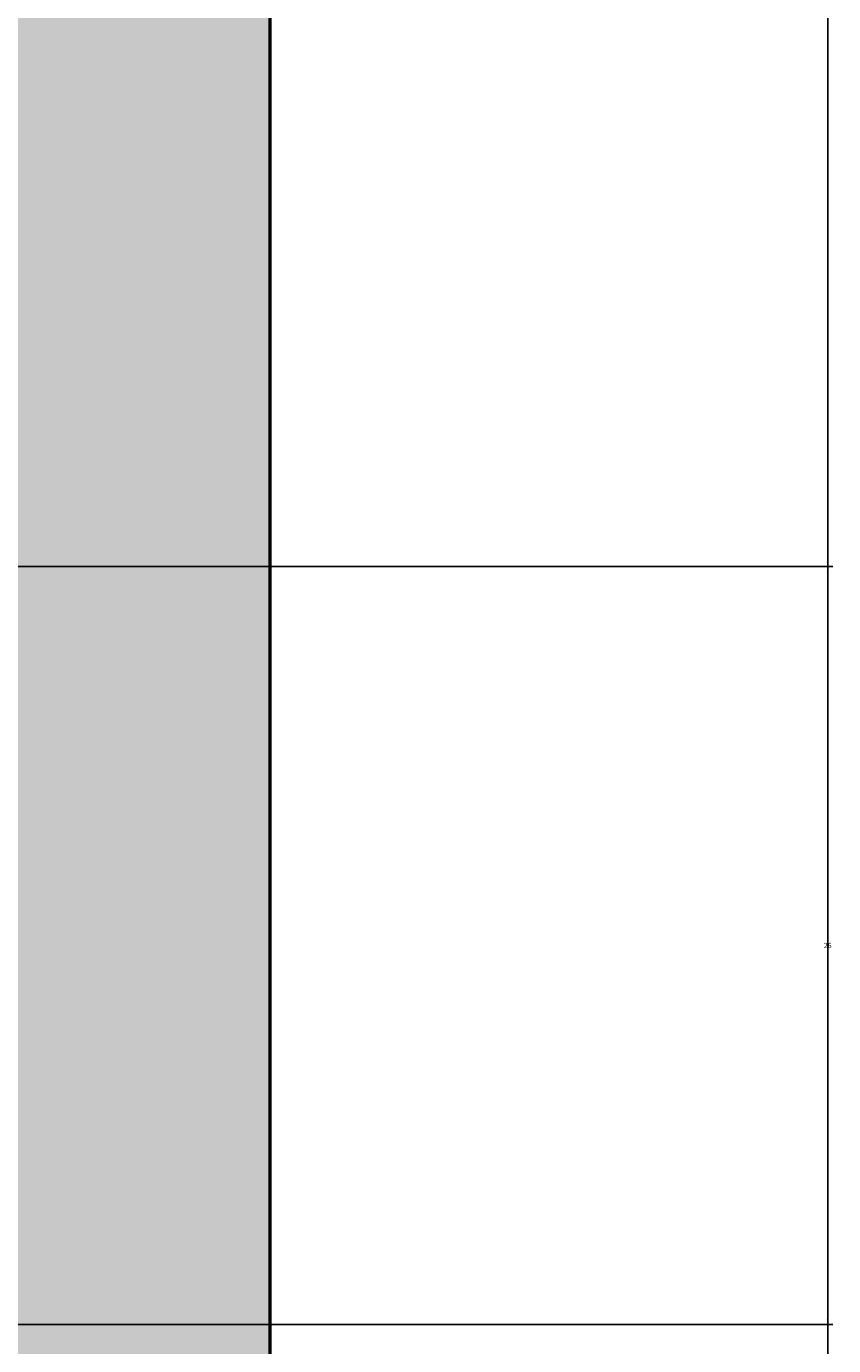
# Model space of a CAD drawing. Units: inches. Extents: x 2307 to 2544, y 2171 to 2540.
# Tile 12 of 52: x 2516 to 2544, y 2199 to 2244. Entities that reach past the tile are written whole.
import ezdxf

# ---------------------------------------------------------------- set-up
doc = ezdxf.new("R2010")
doc.units = ezdxf.units.IN
doc.layers.add('A-ANNO-DIMS', color=2, linetype='Continuous', lineweight=18)
doc.layers.add('A-WALL', color=7, linetype='Continuous', lineweight=50)
doc.layers.add('A-WALL-PATT', color=18, linetype='Continuous', lineweight=13, true_color=0x000000)
doc.styles.get("Standard").update_dxf_attribs({"font": 'arial.ttf'})
doc.dimstyles.get("Standard").update_dxf_attribs({"dimtxt": 0.18, "dimasz": 0.18, "dimexe": 0.18, "dimexo": 0.0625, "dimgap": 0.09, "dimtad": 0, "dimtih": 1, "dimtoh": 1, "dimdec": 4, "dimzin": 0, "dimdsep": 46, "dimtxsty": 'Standard', "dimcen": 0.09, "dimadec": 0, "dimazin": 0, "dimtfac": 1, "dimtdec": 4, "dimtofl": 0, "dimtmove": 0, "dimatfit": 3, "dimfxl": 1, "dimtolj": 1, "dimtzin": 0, "dimarcsym": 0})

# ---------------------------------------------------------------- blocks, each defined once
blk = doc.blocks.new('*D37')
at = {"layer": 'A-ANNO-DIMS', "color": 0, "lineweight": -2, "transparency": 16777216}
for p, q in [((2524.758, 2520.51), (2544.026, 2520.51)), ((2543.846, 2520.33), (2543.846, 2355.692)), ((2543.846, 2190.69), (2543.846, 2355.328)), ((2524.758, 2190.51), (2544.026, 2190.51))]:
    blk.add_line(p, q, dxfattribs=at)
at = {"layer": 'A-ANNO-DIMS', "color": 0, "transparency": 16777216}
for points in [[(2543.816, 2520.33), (2543.876, 2520.33), (2543.846, 2520.51)], [(2543.816, 2190.69), (2543.876, 2190.69), (2543.846, 2190.51)]]:
    blk.add_solid(points, dxfattribs=at)
at = {"layer": 'Defpoints', "color": 0, "transparency": 16777216}
for p in [(2524.696, 2520.51), (2543.846, 2520.51), (2524.696, 2190.51)]:
    blk.add_point(p, dxfattribs=at)
at = {"layer": 'A-ANNO-DIMS', "color": 0, "transparency": 16777216, "insert": (2543.846, 2355.51), "char_height": 0.18, "attachment_point": 5}
blk.add_mtext('\\A1;330', dxfattribs=at)
blk = doc.blocks.new('*D56')
at = {"layer": 'A-ANNO-DIMS', "color": 0, "lineweight": -2, "transparency": 16777216}
for p, q in [((2515.758, 2285.51), (2544.026, 2285.51)), ((2543.846, 2285.33), (2543.846, 2255.691)), ((2543.846, 2225.69), (2543.846, 2255.328)), ((2515.758, 2225.51), (2544.026, 2225.51))]:
    blk.add_line(p, q, dxfattribs=at)
at = {"layer": 'A-ANNO-DIMS', "color": 0, "transparency": 16777216}
for points in [[(2543.816, 2285.33), (2543.876, 2285.33), (2543.846, 2285.51)], [(2543.816, 2225.69), (2543.876, 2225.69), (2543.846, 2225.51)]]:
    blk.add_solid(points, dxfattribs=at)
at = {"layer": 'Defpoints', "color": 0, "transparency": 16777216}
for p in [(2515.696, 2285.51), (2543.846, 2285.51), (2515.696, 2225.51)]:
    blk.add_point(p, dxfattribs=at)
at = {"layer": 'A-ANNO-DIMS', "color": 0, "transparency": 16777216, "insert": (2543.846, 2255.51), "char_height": 0.18, "attachment_point": 5}
blk.add_mtext('\\A1;60', dxfattribs=at)
blk = doc.blocks.new('*D60')
at = {"layer": 'A-ANNO-DIMS', "color": 0, "lineweight": -2, "transparency": 16777216}
for p, q in [((2515.758, 2225.51), (2544.026, 2225.51)), ((2543.846, 2225.33), (2543.846, 2212.691)), ((2543.846, 2199.69), (2543.846, 2212.328)), ((2515.758, 2199.51), (2544.026, 2199.51))]:
    blk.add_line(p, q, dxfattribs=at)
at = {"layer": 'A-ANNO-DIMS', "color": 0, "transparency": 16777216}
for points in [[(2543.816, 2225.33), (2543.876, 2225.33), (2543.846, 2225.51)], [(2543.816, 2199.69), (2543.876, 2199.69), (2543.846, 2199.51)]]:
    blk.add_solid(points, dxfattribs=at)
at = {"layer": 'Defpoints', "color": 0, "transparency": 16777216}
for p in [(2515.696, 2225.51), (2543.846, 2225.51), (2515.696, 2199.51)]:
    blk.add_point(p, dxfattribs=at)
at = {"layer": 'A-ANNO-DIMS', "color": 0, "transparency": 16777216, "insert": (2543.846, 2212.51), "char_height": 0.18, "attachment_point": 5}
blk.add_mtext('\\A1;26', dxfattribs=at)

msp = doc.modelspace()

# ---------------------------------------------------------------- hatches: boundary and pattern name
at = {"layer": 'A-WALL-PATT'}
h = msp.add_hatch(color=256, dxfattribs=at)
h.dxf.hatch_style = 1
h.paths.add_polyline_path([(2433.6935, 2199.5096), (2415.6423, 2199.5096), (2415.6423, 2190.5096), (2433.7832, 2190.5096)], flags=17)
h.paths.add_polyline_path([(2367.6423, 2199.5096), (2335.6958, 2199.5096), (2335.6958, 2307.3983), (2326.6958, 2307.3983), (2326.6958, 2190.5096), (2367.6423, 2190.5096)])
h.paths.add_polyline_path([(2524.6958, 2520.5096), (2496.7832, 2520.5096), (2496.7832, 2515.5149), (2472.7832, 2515.5149), (2472.7832, 2520.5096), (2415.4028, 2520.5096), (2415.4028, 2511.5096), (2451.6958, 2511.5096), (2451.6958, 2439.5096), (2451.6958, 2391.5096), (2445.6958, 2391.5096), (2445.6958, 2387.5096), (2455.6958, 2387.5096), (2455.6958, 2435.5096), (2461.6958, 2435.5096), (2461.6958, 2439.5096), (2455.6958, 2439.5096), (2455.6958, 2511.5096), (2515.6958, 2511.5096), (2515.6958, 2439.5096), (2491.6958, 2439.5096), (2491.6958, 2435.5096), (2515.6958, 2435.5096), (2515.6958, 2319.5096), (2451.6958, 2319.5096), (2451.6958, 2281.5096), (2481.6958, 2281.5096), (2481.6958, 2225.5096), (2485.6958, 2225.5096), (2485.6958, 2285.5096), (2455.6958, 2285.5096), (2455.6958, 2315.5096), (2515.6958, 2315.5096), (2515.6958, 2199.5096), (2469.6952, 2199.5096), (2469.785, 2190.5096), (2524.6958, 2190.5096)])

# ---------------------------------------------------------------- linework, layer by layer
at = {"layer": 'A-WALL'}
msp.add_lwpolyline([(2433.7832, 2190.5096), (2326.6958, 2190.5096), (2326.6958, 2520.5096), (2524.6958, 2520.5096), (2524.6958, 2190.5096), (2469.785, 2190.5096)], dxfattribs=at)

# ---------------------------------------------------------------- dimensions: what is measured, and where the dimension line sits
at = {"layer": 'A-ANNO-DIMS'}
for base, p1, p2, picture, middle in [((2543.8458, 2520.5096), (2524.6958, 2190.5096), (2524.6958, 2520.5096), '*D37', (2543.8458, 2355.5096)), ((2543.8458, 2285.5096), (2515.6958, 2225.5096), (2515.6958, 2285.5096), '*D56', (2543.8458, 2255.5096)), ((2543.8458, 2225.5096), (2515.6958, 2199.5096), (2515.6958, 2225.5096), '*D60', (2543.8458, 2212.5096))]:
    dim = msp.add_linear_dim(base=base, p1=p1, p2=p2, angle=90, dimstyle='Standard', override={"dimdec": 0, "dimlfac": 1, "dimrnd": 0, "dimzin": 0, "dimdsep": 46, "dimlunit": 2}, dxfattribs=at)
    dim.commit()
    dim.dimension.update_dxf_attribs({"geometry": picture, "text_midpoint": middle})

doc.saveas('drawing.dxf')
